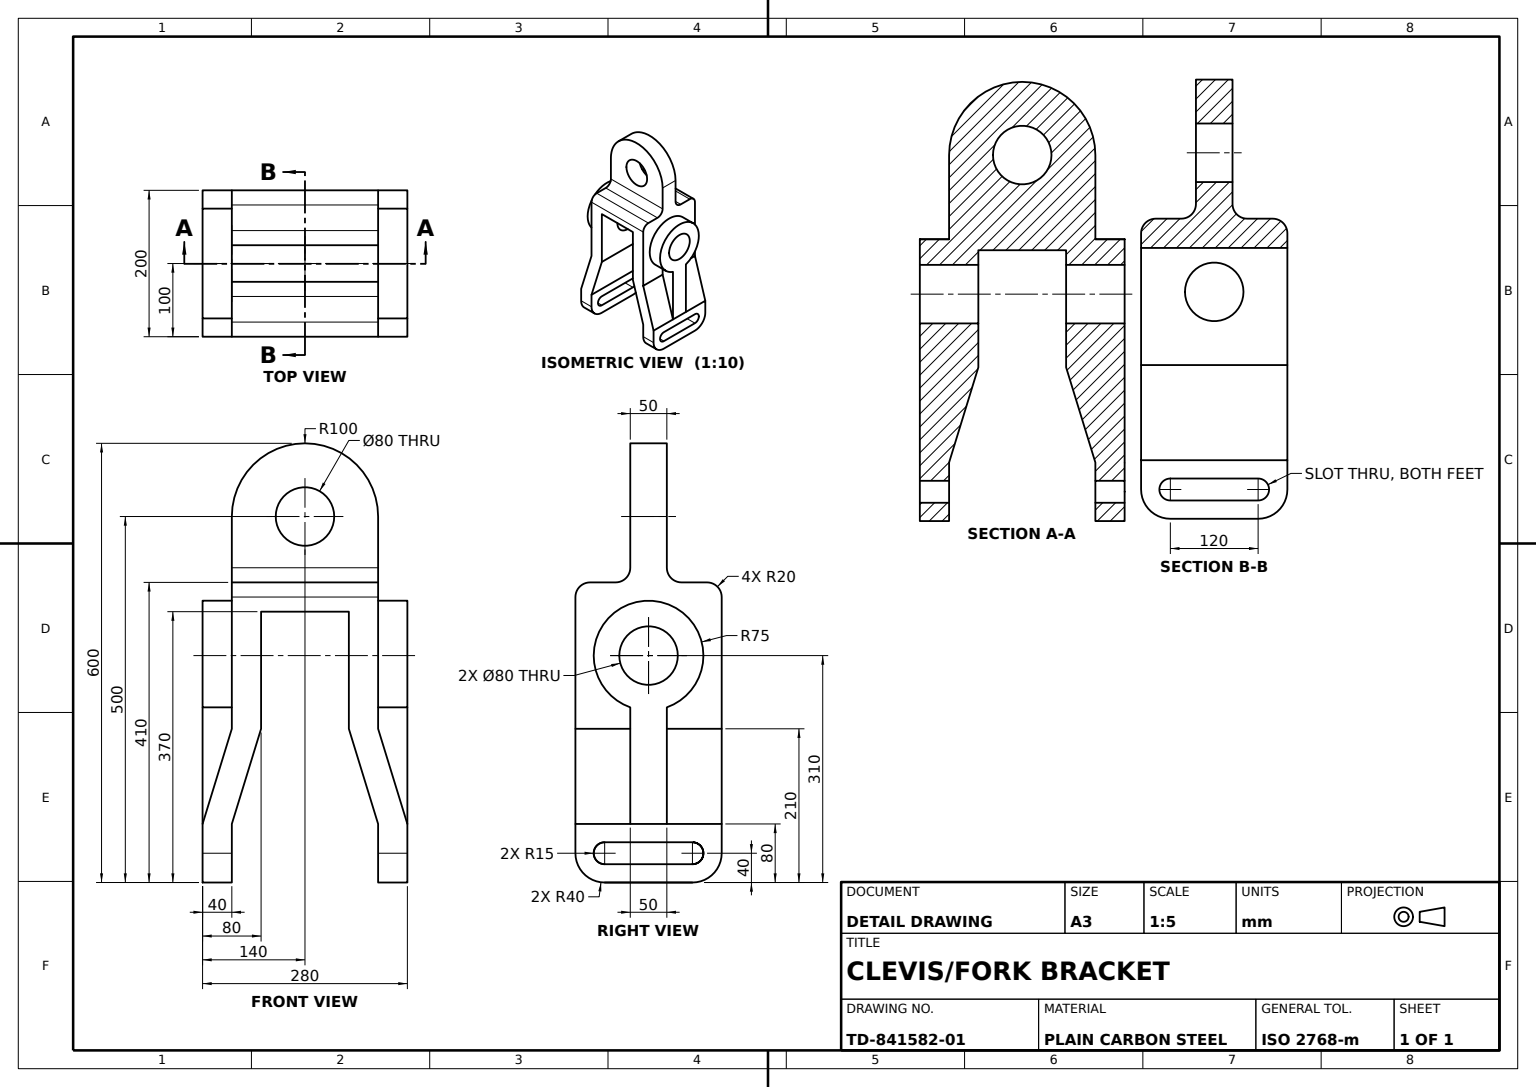
from build123d import *

# Parameters (mm, degrees)
FORK_BODY_DEPTH         = 200
SIDE_BOSS_A_SKETCH_R    = 40
SIDE_BOSS_A_DEPTH       = 40
SIDE_START              = 40
SIDE_BOSS_B_SKETCH_R    = 40
SIDE_BOSS_B_DEPTH       = 40
PIVOT_BORE_SKETCH_R     = 40
PIVOT_BORE_80_DEPTH     = 516.460958754
TOP_LUG_SKETCH_R        = 40
TOP_LUG_DEPTH           = 25
TOP_LUG_BLEND_R20_R     = 20
FORK_FILLET_R40_A_R     = 40
FORK_FILLET_R40_B_R     = 40
FORK_FILLET_R40_C_R     = 40
FORK_FILLET_R40_D_R     = 40
FOOT_SLOTS_15X120_DEPTH = 536.253402042


with BuildPart() as part:
    # Fork Profile Sketch → Fork Body (new body)
    with BuildSketch(Plane.XY):
        Polygon((0, 0), (-100, 0), (-100, -200), (-139.993222056, -330), (-139.993222056, -410), (-99.993222056, -410), (-99.993222056, -330), (-60, -200), (-60, -40), (60, -40), (60, -200), (99.993222056, -330), (99.993222056, -410), (139.993222056, -410), (139.993222056, -330), (100, -200), (100, 0), align=None)
    extrude(amount=-FORK_BODY_DEPTH)

    # Side Boss A Sketch → Side Boss A (add)
    with BuildSketch(Plane(origin=(140, 0, 0), x_dir=(0, 0, -1), z_dir=(1, 0, 0))):
        with BuildLine():
            Line((75, -170.710678119), (75, -330))
            Line((75, -330), (125, -330))
            Line((125, -330), (125, -170.710678119))
            ThreePointArc((125, -170.710678119), (100, -25), (75, -170.710678119))
        make_face()
        with Locations((100, -100)):
            Circle(SIDE_BOSS_A_SKETCH_R, mode=Mode.SUBTRACT)
    extrude(amount=-SIDE_BOSS_A_DEPTH)

    # Side Boss B Sketch → Side Boss B (add)
    with BuildSketch(Plane(origin=(-140, 0, 0), x_dir=(0, 0, -1), z_dir=(1, 0, 0)).offset(SIDE_START)):
        with BuildLine():
            Line((125, -170.710678119), (125, -330))
            Line((125, -330), (75, -330))
            Line((75, -330), (75, -170.710678119))
            ThreePointArc((75, -170.710678119), (100, -25), (125, -170.710678119))
        make_face()
        with Locations((100, -100)):
            Circle(SIDE_BOSS_B_SKETCH_R, mode=Mode.SUBTRACT)
    extrude(amount=-SIDE_BOSS_B_DEPTH)

    # Pivot Bore Sketch → Pivot Bore Ø80 (cut, through all)
    with BuildSketch(Plane(origin=(100, 0, 0), x_dir=(0, 0, -1), z_dir=(1, 0, 0))):
        with Locations((100, -100)):
            Circle(PIVOT_BORE_SKETCH_R)
    extrude(amount=-PIVOT_BORE_80_DEPTH, mode=Mode.SUBTRACT)

    # Top Lug Sketch → Top Lug (add, symmetric)
    with BuildSketch(Plane.XY.offset(-100)):
        with BuildLine():
            Line((-100, 90), (-100, 0))
            Line((-100, 0), (100, 0))
            Line((100, 0), (100, 90))
            ThreePointArc((100, 90), (0, 190), (-100, 90))
        make_face()
        with Locations((0, 90)):
            Circle(TOP_LUG_SKETCH_R, mode=Mode.SUBTRACT)
    extrude(amount=TOP_LUG_DEPTH, both=True)

    # Top Lug Blend R20
    top_lug_blend_r20_edges = [part.edges().sort_by_distance(p)[0] for p in [
        (0, 0, -75),
        (0, 0, -125),
        (0, 0, 0),
        (0, 0, -200),
    ]]
    fillet(top_lug_blend_r20_edges, radius=TOP_LUG_BLEND_R20_R)

    # Fork Fillet R40 A
    fork_fillet_r40_a_edges = [part.edges().sort_by_distance(p)[0] for p in [
        (119.993222056, -410, 0),
    ]]
    fillet(fork_fillet_r40_a_edges, radius=FORK_FILLET_R40_A_R)

    # Fork Fillet R40 B
    fork_fillet_r40_b_edges = [part.edges().sort_by_distance(p)[0] for p in [
        (119.993222056, -410, -200),
    ]]
    fillet(fork_fillet_r40_b_edges, radius=FORK_FILLET_R40_B_R)

    # Fork Fillet R40 C
    fork_fillet_r40_c_edges = [part.edges().sort_by_distance(p)[0] for p in [
        (-119.993222056, -410, 0),
    ]]
    fillet(fork_fillet_r40_c_edges, radius=FORK_FILLET_R40_C_R)

    # Fork Fillet R40 D
    fork_fillet_r40_d_edges = [part.edges().sort_by_distance(p)[0] for p in [
        (-119.993222056, -410, -200),
    ]]
    fillet(fork_fillet_r40_d_edges, radius=FORK_FILLET_R40_D_R)

    # Foot Slot Sketch → Foot Slots 15x120 (cut, through all)
    with BuildSketch(Plane(origin=(139.993222056, 0, 0), x_dir=(0, 0, -1), z_dir=(1, 0, 0))):
        with BuildLine():
            Line((40, -355), (160, -355))
            ThreePointArc((160, -355), (175, -370), (160, -385))
            Line((160, -385), (40, -385))
            ThreePointArc((40, -385), (25, -370), (40, -355))
        make_face()
    extrude(amount=-FOOT_SLOTS_15X120_DEPTH, mode=Mode.SUBTRACT)


solid = part.part
